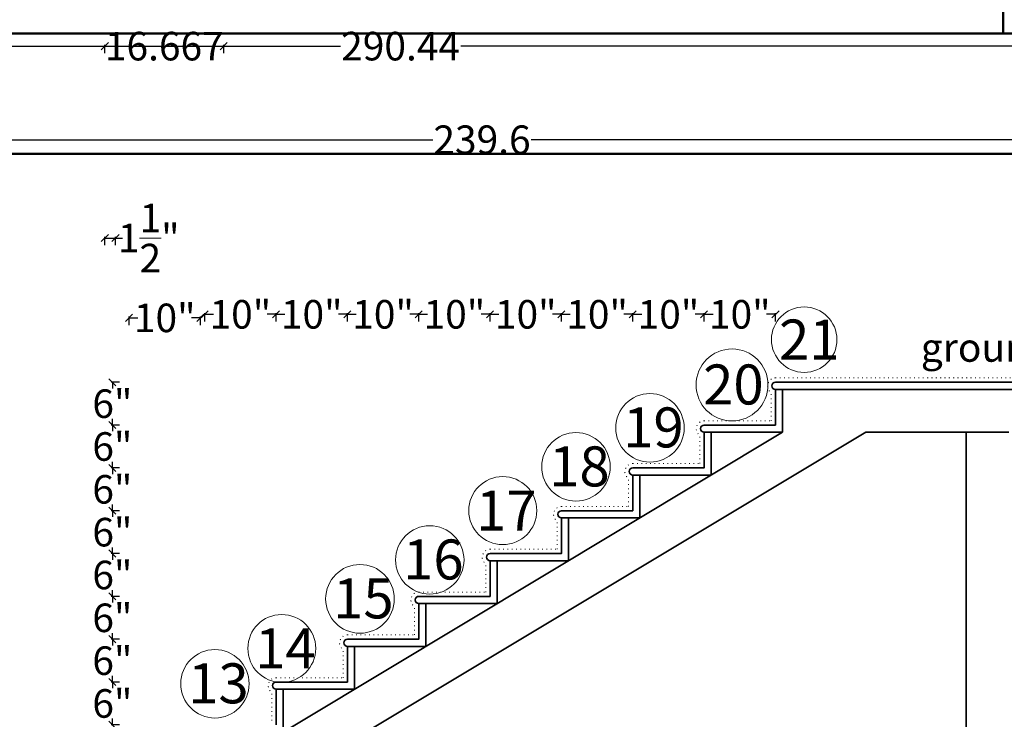
# Model space of a CAD drawing. Units: inches. Extents: x -60 to 284, y -245 to 257.
# Tile 4 of 10: x 55 to 193, y -86 to 12. Entities that reach past the tile are written whole.
import ezdxf

# ---------------------------------------------------------------- set-up
doc = ezdxf.new("R2010")
doc.units = ezdxf.units.IN
doc.header["$LTSCALE"] = 0.8
doc.header["$MEASUREMENT"] = 0
doc.linetypes.add('DOT', pattern=[6.35, 0, -6.35])
for name, color, linetype, lineweight in [('A-ANNO-DIMS', 2, 'Continuous', 18), ('A-ANNO-SYMB', 3, 'Continuous', 18), ('A-ANNO-TEXT', 3, 'Continuous', 18), ('A-ANNO-TTLB', 7, 'Continuous', 50), ('A-SECT', 7, 'Continuous', 35), ('A-SECT-OVHD', 8, 'DOT', 18), ('A-WALL', 7, 'Continuous', 50)]:
    doc.layers.add(name, color=color, linetype=linetype, lineweight=lineweight)
doc.styles.get("Standard").update_dxf_attribs({"font": 'arial.ttf'})
doc.dimstyles.get("Standard").update_dxf_attribs({"dimtxt": 4, "dimasz": 1, "dimexe": 0.18, "dimexo": 0.0625, "dimgap": 0.09, "dimtad": 0, "dimtih": 1, "dimtoh": 1, "dimzin": 0, "dimdsep": 46, "dimlunit": 4, "dimtxsty": 'Standard', "dimblk": 'OBLIQUE', "dimcen": 0.09, "dimadec": 0, "dimazin": 0, "dimtfac": 1, "dimtofl": 0, "dimtmove": 0, "dimatfit": 3, "dimfxl": 1, "dimfxlon": 1, "dimtolj": 1, "dimtzin": 0, "dimarcsym": 0})

# ---------------------------------------------------------------- blocks, each defined once
blk = doc.blocks.new('_Oblique')
at = {"color": 0, "linetype": 'ByBlock', "lineweight": -2}
blk.add_line((-0.5, -0.5), (0.5, 0.5), dxfattribs=at)
blk = doc.blocks.new('*D51')
at = {"layer": 'A-ANNO-DIMS', "color": 0, "lineweight": -2, "ltscale": 0.8, "transparency": 16777216}
for p, q in [((81.01, -30.69), (81.01, -29.51)), ((81.01, -29.69), (82.26, -29.69)), ((91.01, -29.69), (89.77, -29.69)), ((91.01, -30.69), (91.01, -29.51))]:
    blk.add_line(p, q, dxfattribs=at)
at = {"layer": 'Defpoints', "color": 0, "ltscale": 0.8, "transparency": 16777216}
for p in [(91.01, -29.69), (81.01, -87.21), (91.01, -87.21)]:
    blk.add_point(p, dxfattribs=at)
at = {"layer": 'A-ANNO-DIMS', "color": 0, "lineweight": -2, "ltscale": 0.8, "transparency": 16777216, "rotation": 180}
blk.add_blockref('_Oblique', (81.01, -29.69), dxfattribs=at)
at = {"layer": 'A-ANNO-DIMS', "color": 0, "lineweight": -2, "ltscale": 0.8, "transparency": 16777216}
blk.add_blockref('_Oblique', (91.01, -29.69), dxfattribs=at)
at = {"layer": 'A-ANNO-DIMS', "color": 0, "ltscale": 0.8, "transparency": 16777216, "insert": (86.01, -29.69), "char_height": 4, "attachment_point": 5}
blk.add_mtext('\\A1;10"', dxfattribs=at)
blk = doc.blocks.new('*D52')
at = {"layer": 'A-ANNO-DIMS', "color": 0, "lineweight": -2, "ltscale": 0.8, "transparency": 16777216}
for p, q in [((91.01, -30.69), (91.01, -29.51)), ((91.01, -29.69), (92.26, -29.69)), ((101.01, -29.69), (99.77, -29.69)), ((101.01, -30.69), (101.01, -29.51))]:
    blk.add_line(p, q, dxfattribs=at)
at = {"layer": 'Defpoints', "color": 0, "ltscale": 0.8, "transparency": 16777216}
for p in [(101.01, -29.69), (91.01, -81.21), (101.01, -81.21)]:
    blk.add_point(p, dxfattribs=at)
at = {"layer": 'A-ANNO-DIMS', "color": 0, "lineweight": -2, "ltscale": 0.8, "transparency": 16777216, "rotation": 180}
blk.add_blockref('_Oblique', (91.01, -29.69), dxfattribs=at)
at = {"layer": 'A-ANNO-DIMS', "color": 0, "lineweight": -2, "ltscale": 0.8, "transparency": 16777216}
blk.add_blockref('_Oblique', (101.01, -29.69), dxfattribs=at)
at = {"layer": 'A-ANNO-DIMS', "color": 0, "ltscale": 0.8, "transparency": 16777216, "insert": (96.01, -29.69), "char_height": 4, "attachment_point": 5}
blk.add_mtext('\\A1;10"', dxfattribs=at)
blk = doc.blocks.new('*D53')
at = {"layer": 'A-ANNO-DIMS', "color": 0, "lineweight": -2, "ltscale": 0.8, "transparency": 16777216}
for p, q in [((101.01, -30.69), (101.01, -29.51)), ((101.01, -29.69), (102.26, -29.69)), ((111.01, -29.69), (109.77, -29.69)), ((111.01, -30.69), (111.01, -29.51))]:
    blk.add_line(p, q, dxfattribs=at)
at = {"layer": 'Defpoints', "color": 0, "ltscale": 0.8, "transparency": 16777216}
for p in [(111.01, -29.69), (101.01, -75.21), (111.01, -75.21)]:
    blk.add_point(p, dxfattribs=at)
at = {"layer": 'A-ANNO-DIMS', "color": 0, "lineweight": -2, "ltscale": 0.8, "transparency": 16777216, "rotation": 180}
blk.add_blockref('_Oblique', (101.01, -29.69), dxfattribs=at)
at = {"layer": 'A-ANNO-DIMS', "color": 0, "lineweight": -2, "ltscale": 0.8, "transparency": 16777216}
blk.add_blockref('_Oblique', (111.01, -29.69), dxfattribs=at)
at = {"layer": 'A-ANNO-DIMS', "color": 0, "ltscale": 0.8, "transparency": 16777216, "insert": (106.01, -29.69), "char_height": 4, "attachment_point": 5}
blk.add_mtext('\\A1;10"', dxfattribs=at)
blk = doc.blocks.new('*D54')
at = {"layer": 'A-ANNO-DIMS', "color": 0, "lineweight": -2, "ltscale": 0.8, "transparency": 16777216}
for p, q in [((111.01, -30.69), (111.01, -29.51)), ((111.01, -29.69), (112.26, -29.69)), ((121.01, -29.69), (119.77, -29.69)), ((121.01, -30.69), (121.01, -29.51))]:
    blk.add_line(p, q, dxfattribs=at)
at = {"layer": 'Defpoints', "color": 0, "ltscale": 0.8, "transparency": 16777216}
for p in [(121.01, -29.69), (111.01, -69.21), (121.01, -69.21)]:
    blk.add_point(p, dxfattribs=at)
at = {"layer": 'A-ANNO-DIMS', "color": 0, "lineweight": -2, "ltscale": 0.8, "transparency": 16777216, "rotation": 180}
blk.add_blockref('_Oblique', (111.01, -29.69), dxfattribs=at)
at = {"layer": 'A-ANNO-DIMS', "color": 0, "lineweight": -2, "ltscale": 0.8, "transparency": 16777216}
blk.add_blockref('_Oblique', (121.01, -29.69), dxfattribs=at)
at = {"layer": 'A-ANNO-DIMS', "color": 0, "ltscale": 0.8, "transparency": 16777216, "insert": (116.01, -29.69), "char_height": 4, "attachment_point": 5}
blk.add_mtext('\\A1;10"', dxfattribs=at)
blk = doc.blocks.new('*D55')
at = {"layer": 'A-ANNO-DIMS', "color": 0, "lineweight": -2, "ltscale": 0.8, "transparency": 16777216}
for p, q in [((121.01, -30.69), (121.01, -29.51)), ((121.01, -29.69), (122.26, -29.69)), ((131.01, -29.69), (129.77, -29.69)), ((131.01, -30.69), (131.01, -29.51))]:
    blk.add_line(p, q, dxfattribs=at)
at = {"layer": 'Defpoints', "color": 0, "ltscale": 0.8, "transparency": 16777216}
for p in [(131.01, -29.69), (121.01, -63.21), (131.01, -63.21)]:
    blk.add_point(p, dxfattribs=at)
at = {"layer": 'A-ANNO-DIMS', "color": 0, "lineweight": -2, "ltscale": 0.8, "transparency": 16777216, "rotation": 180}
blk.add_blockref('_Oblique', (121.01, -29.69), dxfattribs=at)
at = {"layer": 'A-ANNO-DIMS', "color": 0, "lineweight": -2, "ltscale": 0.8, "transparency": 16777216}
blk.add_blockref('_Oblique', (131.01, -29.69), dxfattribs=at)
at = {"layer": 'A-ANNO-DIMS', "color": 0, "ltscale": 0.8, "transparency": 16777216, "insert": (126.01, -29.69), "char_height": 4, "attachment_point": 5}
blk.add_mtext('\\A1;10"', dxfattribs=at)
blk = doc.blocks.new('*D56')
at = {"layer": 'A-ANNO-DIMS', "color": 0, "lineweight": -2, "ltscale": 0.8, "transparency": 16777216}
for p, q in [((131.01, -30.69), (131.01, -29.51)), ((131.01, -29.69), (132.26, -29.69)), ((141.01, -29.69), (139.77, -29.69)), ((141.01, -30.69), (141.01, -29.51))]:
    blk.add_line(p, q, dxfattribs=at)
at = {"layer": 'Defpoints', "color": 0, "ltscale": 0.8, "transparency": 16777216}
for p in [(141.01, -29.69), (131.01, -57.21), (141.01, -57.21)]:
    blk.add_point(p, dxfattribs=at)
at = {"layer": 'A-ANNO-DIMS', "color": 0, "lineweight": -2, "ltscale": 0.8, "transparency": 16777216, "rotation": 180}
blk.add_blockref('_Oblique', (131.01, -29.69), dxfattribs=at)
at = {"layer": 'A-ANNO-DIMS', "color": 0, "lineweight": -2, "ltscale": 0.8, "transparency": 16777216}
blk.add_blockref('_Oblique', (141.01, -29.69), dxfattribs=at)
at = {"layer": 'A-ANNO-DIMS', "color": 0, "ltscale": 0.8, "transparency": 16777216, "insert": (136.01, -29.69), "char_height": 4, "attachment_point": 5}
blk.add_mtext('\\A1;10"', dxfattribs=at)
blk = doc.blocks.new('*D57')
at = {"layer": 'A-ANNO-DIMS', "color": 0, "lineweight": -2, "ltscale": 0.8, "transparency": 16777216}
for p, q in [((141.01, -30.69), (141.01, -29.51)), ((141.01, -29.69), (142.26, -29.69)), ((151.01, -29.69), (149.77, -29.69)), ((151.01, -30.69), (151.01, -29.51))]:
    blk.add_line(p, q, dxfattribs=at)
at = {"layer": 'Defpoints', "color": 0, "ltscale": 0.8, "transparency": 16777216}
for p in [(151.01, -29.69), (141.01, -51.21), (151.01, -51.21)]:
    blk.add_point(p, dxfattribs=at)
at = {"layer": 'A-ANNO-DIMS', "color": 0, "lineweight": -2, "ltscale": 0.8, "transparency": 16777216, "rotation": 180}
blk.add_blockref('_Oblique', (141.01, -29.69), dxfattribs=at)
at = {"layer": 'A-ANNO-DIMS', "color": 0, "lineweight": -2, "ltscale": 0.8, "transparency": 16777216}
blk.add_blockref('_Oblique', (151.01, -29.69), dxfattribs=at)
at = {"layer": 'A-ANNO-DIMS', "color": 0, "ltscale": 0.8, "transparency": 16777216, "insert": (146.01, -29.69), "char_height": 4, "attachment_point": 5}
blk.add_mtext('\\A1;10"', dxfattribs=at)
blk = doc.blocks.new('*D58')
at = {"layer": 'A-ANNO-DIMS', "color": 0, "lineweight": -2, "ltscale": 0.8, "transparency": 16777216}
for p, q in [((151.01, -30.69), (151.01, -29.51)), ((151.01, -29.69), (152.26, -29.69)), ((161.01, -29.69), (159.77, -29.69)), ((161.01, -30.69), (161.01, -29.51))]:
    blk.add_line(p, q, dxfattribs=at)
at = {"layer": 'Defpoints', "color": 0, "ltscale": 0.8, "transparency": 16777216}
for p in [(161.01, -29.69), (151.01, -45.21), (161.01, -45.21)]:
    blk.add_point(p, dxfattribs=at)
at = {"layer": 'A-ANNO-DIMS', "color": 0, "lineweight": -2, "ltscale": 0.8, "transparency": 16777216, "rotation": 180}
blk.add_blockref('_Oblique', (151.01, -29.69), dxfattribs=at)
at = {"layer": 'A-ANNO-DIMS', "color": 0, "lineweight": -2, "ltscale": 0.8, "transparency": 16777216}
blk.add_blockref('_Oblique', (161.01, -29.69), dxfattribs=at)
at = {"layer": 'A-ANNO-DIMS', "color": 0, "ltscale": 0.8, "transparency": 16777216, "insert": (156.01, -29.69), "char_height": 4, "attachment_point": 5}
blk.add_mtext('\\A1;10"', dxfattribs=at)
blk = doc.blocks.new('*D60')
at = {"layer": 'A-ANNO-DIMS', "color": 0, "lineweight": -2, "ltscale": 0.8, "transparency": 16777216}
for p, q in [((69.07, -81.21), (67.89, -81.21)), ((68.07, -81.21), (68.07, -82.08)), ((68.07, -87.21), (68.07, -86.34)), ((69.07, -87.21), (67.89, -87.21))]:
    blk.add_line(p, q, dxfattribs=at)
at = {"layer": 'Defpoints', "color": 0, "ltscale": 0.8, "transparency": 16777216}
for p in [(68.07, -81.21), (91.01, -81.21), (91.01, -87.21)]:
    blk.add_point(p, dxfattribs=at)
at = {"layer": 'A-ANNO-DIMS', "color": 0, "lineweight": -2, "ltscale": 0.8, "transparency": 16777216}
for p, rotation in [((68.07, -81.21), 90), ((68.07, -87.21), 270)]:
    blk.add_blockref('_Oblique', p, dxfattribs=dict(at, rotation=rotation))
at = {"layer": 'A-ANNO-DIMS', "color": 0, "ltscale": 0.8, "transparency": 16777216, "insert": (68.07, -84.21), "char_height": 4, "attachment_point": 5}
blk.add_mtext('\\A1;6"', dxfattribs=at)
blk = doc.blocks.new('*D61')
at = {"layer": 'A-ANNO-DIMS', "color": 0, "lineweight": -2, "ltscale": 0.8, "transparency": 16777216}
for p, q in [((69.07, -75.21), (67.89, -75.21)), ((68.07, -75.21), (68.07, -76.08)), ((69.07, -81.21), (67.89, -81.21)), ((68.07, -81.21), (68.07, -80.34))]:
    blk.add_line(p, q, dxfattribs=at)
at = {"layer": 'Defpoints', "color": 0, "ltscale": 0.8, "transparency": 16777216}
for p in [(68.07, -75.21), (101.01, -75.21), (101.01, -81.21)]:
    blk.add_point(p, dxfattribs=at)
at = {"layer": 'A-ANNO-DIMS', "color": 0, "lineweight": -2, "ltscale": 0.8, "transparency": 16777216}
for p, rotation in [((68.07, -75.21), 90), ((68.07, -81.21), 270)]:
    blk.add_blockref('_Oblique', p, dxfattribs=dict(at, rotation=rotation))
at = {"layer": 'A-ANNO-DIMS', "color": 0, "ltscale": 0.8, "transparency": 16777216, "insert": (68.07, -78.21), "char_height": 4, "attachment_point": 5}
blk.add_mtext('\\A1;6"', dxfattribs=at)
blk = doc.blocks.new('*D62')
at = {"layer": 'A-ANNO-DIMS', "color": 0, "lineweight": -2, "ltscale": 0.8, "transparency": 16777216}
for p, q in [((69.07, -69.21), (67.89, -69.21)), ((68.07, -69.21), (68.07, -70.08)), ((68.07, -75.21), (68.07, -74.34)), ((69.07, -75.21), (67.89, -75.21))]:
    blk.add_line(p, q, dxfattribs=at)
at = {"layer": 'Defpoints', "color": 0, "ltscale": 0.8, "transparency": 16777216}
for p in [(68.07, -69.21), (111.01, -69.21), (111.01, -75.21)]:
    blk.add_point(p, dxfattribs=at)
at = {"layer": 'A-ANNO-DIMS', "color": 0, "lineweight": -2, "ltscale": 0.8, "transparency": 16777216}
for p, rotation in [((68.07, -69.21), 90), ((68.07, -75.21), 270)]:
    blk.add_blockref('_Oblique', p, dxfattribs=dict(at, rotation=rotation))
at = {"layer": 'A-ANNO-DIMS', "color": 0, "ltscale": 0.8, "transparency": 16777216, "insert": (68.07, -72.21), "char_height": 4, "attachment_point": 5}
blk.add_mtext('\\A1;6"', dxfattribs=at)
blk = doc.blocks.new('*D63')
at = {"layer": 'A-ANNO-DIMS', "color": 0, "lineweight": -2, "ltscale": 0.8, "transparency": 16777216}
for p, q in [((69.07, -63.21), (67.89, -63.21)), ((68.07, -63.21), (68.07, -64.08)), ((68.07, -69.21), (68.07, -68.34)), ((69.07, -69.21), (67.89, -69.21))]:
    blk.add_line(p, q, dxfattribs=at)
at = {"layer": 'Defpoints', "color": 0, "ltscale": 0.8, "transparency": 16777216}
for p in [(68.07, -63.21), (121.01, -63.21), (121.01, -69.21)]:
    blk.add_point(p, dxfattribs=at)
at = {"layer": 'A-ANNO-DIMS', "color": 0, "lineweight": -2, "ltscale": 0.8, "transparency": 16777216}
for p, rotation in [((68.07, -63.21), 90), ((68.07, -69.21), 270)]:
    blk.add_blockref('_Oblique', p, dxfattribs=dict(at, rotation=rotation))
at = {"layer": 'A-ANNO-DIMS', "color": 0, "ltscale": 0.8, "transparency": 16777216, "insert": (68.07, -66.21), "char_height": 4, "attachment_point": 5}
blk.add_mtext('\\A1;6"', dxfattribs=at)
blk = doc.blocks.new('*D64')
at = {"layer": 'A-ANNO-DIMS', "color": 0, "lineweight": -2, "ltscale": 0.8, "transparency": 16777216}
for p, q in [((69.07, -57.21), (67.89, -57.21)), ((68.07, -57.21), (68.07, -58.08)), ((69.07, -63.21), (67.89, -63.21)), ((68.07, -63.21), (68.07, -62.34))]:
    blk.add_line(p, q, dxfattribs=at)
at = {"layer": 'Defpoints', "color": 0, "ltscale": 0.8, "transparency": 16777216}
for p in [(68.07, -57.21), (131.01, -57.21), (131.01, -63.21)]:
    blk.add_point(p, dxfattribs=at)
at = {"layer": 'A-ANNO-DIMS', "color": 0, "lineweight": -2, "ltscale": 0.8, "transparency": 16777216}
for p, rotation in [((68.07, -57.21), 90), ((68.07, -63.21), 270)]:
    blk.add_blockref('_Oblique', p, dxfattribs=dict(at, rotation=rotation))
at = {"layer": 'A-ANNO-DIMS', "color": 0, "ltscale": 0.8, "transparency": 16777216, "insert": (68.07, -60.21), "char_height": 4, "attachment_point": 5}
blk.add_mtext('\\A1;6"', dxfattribs=at)
blk = doc.blocks.new('*D65')
at = {"layer": 'A-ANNO-DIMS', "color": 0, "lineweight": -2, "ltscale": 0.8, "transparency": 16777216}
for p, q in [((69.07, -51.21), (67.89, -51.21)), ((68.07, -51.21), (68.07, -52.08)), ((68.07, -57.21), (68.07, -56.34)), ((69.07, -57.21), (67.89, -57.21))]:
    blk.add_line(p, q, dxfattribs=at)
at = {"layer": 'Defpoints', "color": 0, "ltscale": 0.8, "transparency": 16777216}
for p in [(68.07, -51.21), (141.01, -51.21), (141.01, -57.21)]:
    blk.add_point(p, dxfattribs=at)
at = {"layer": 'A-ANNO-DIMS', "color": 0, "lineweight": -2, "ltscale": 0.8, "transparency": 16777216}
for p, rotation in [((68.07, -51.21), 90), ((68.07, -57.21), 270)]:
    blk.add_blockref('_Oblique', p, dxfattribs=dict(at, rotation=rotation))
at = {"layer": 'A-ANNO-DIMS', "color": 0, "ltscale": 0.8, "transparency": 16777216, "insert": (68.07, -54.21), "char_height": 4, "attachment_point": 5}
blk.add_mtext('\\A1;6"', dxfattribs=at)
blk = doc.blocks.new('*D66')
at = {"layer": 'A-ANNO-DIMS', "color": 0, "lineweight": -2, "ltscale": 0.8, "transparency": 16777216}
for p, q in [((69.07, -45.21), (67.89, -45.21)), ((68.07, -45.21), (68.07, -46.08)), ((68.07, -51.21), (68.07, -50.34)), ((69.07, -51.21), (67.89, -51.21))]:
    blk.add_line(p, q, dxfattribs=at)
at = {"layer": 'Defpoints', "color": 0, "ltscale": 0.8, "transparency": 16777216}
for p in [(68.07, -45.21), (151.01, -45.21), (151.01, -51.21)]:
    blk.add_point(p, dxfattribs=at)
at = {"layer": 'A-ANNO-DIMS', "color": 0, "lineweight": -2, "ltscale": 0.8, "transparency": 16777216}
for p, rotation in [((68.07, -45.21), 90), ((68.07, -51.21), 270)]:
    blk.add_blockref('_Oblique', p, dxfattribs=dict(at, rotation=rotation))
at = {"layer": 'A-ANNO-DIMS', "color": 0, "ltscale": 0.8, "transparency": 16777216, "insert": (68.07, -48.21), "char_height": 4, "attachment_point": 5}
blk.add_mtext('\\A1;6"', dxfattribs=at)
blk = doc.blocks.new('*D67')
at = {"layer": 'A-ANNO-DIMS', "color": 0, "lineweight": -2, "ltscale": 0.8, "transparency": 16777216}
for p, q in [((69.07, -39.21), (67.89, -39.21)), ((68.07, -39.21), (68.07, -40.08)), ((69.07, -45.21), (67.89, -45.21)), ((68.07, -45.21), (68.07, -44.34))]:
    blk.add_line(p, q, dxfattribs=at)
at = {"layer": 'Defpoints', "color": 0, "ltscale": 0.8, "transparency": 16777216}
for p in [(68.07, -39.21), (161.01, -39.21), (161.01, -45.21)]:
    blk.add_point(p, dxfattribs=at)
at = {"layer": 'A-ANNO-DIMS', "color": 0, "lineweight": -2, "ltscale": 0.8, "transparency": 16777216}
for p, rotation in [((68.07, -39.21), 90), ((68.07, -45.21), 270)]:
    blk.add_blockref('_Oblique', p, dxfattribs=dict(at, rotation=rotation))
at = {"layer": 'A-ANNO-DIMS', "color": 0, "ltscale": 0.8, "transparency": 16777216, "insert": (68.07, -42.21), "char_height": 4, "attachment_point": 5}
blk.add_mtext('\\A1;6"', dxfattribs=at)
blk = doc.blocks.new('*D72')
at = {"layer": 'A-ANNO-DIMS', "color": 0, "lineweight": -2, "ltscale": 0.8, "transparency": 16777216}
for p, q in [((67.01, -20.01), (67.01, -18.83)), ((67.01, -19.01), (68.51, -19.01)), ((68.51, -20.01), (68.51, -18.83)), ((68.51, -19.01), (69.51, -19.01))]:
    blk.add_line(p, q, dxfattribs=at)
at = {"layer": 'Defpoints', "color": 0, "ltscale": 0.8, "transparency": 16777216}
for p in [(68.51, -19.01), (67.01, -93.21), (68.51, -93.21)]:
    blk.add_point(p, dxfattribs=at)
at = {"layer": 'A-ANNO-DIMS', "color": 0, "lineweight": -2, "ltscale": 0.8, "transparency": 16777216, "rotation": 180}
blk.add_blockref('_Oblique', (67.01, -19.01), dxfattribs=at)
at = {"layer": 'A-ANNO-DIMS', "color": 0, "lineweight": -2, "ltscale": 0.8, "transparency": 16777216}
blk.add_blockref('_Oblique', (68.51, -19.01), dxfattribs=at)
at = {"layer": 'A-ANNO-DIMS', "color": 0, "ltscale": 0.8, "transparency": 16777216, "insert": (73.17, -19.01), "char_height": 4, "attachment_point": 5}
blk.add_mtext('\\A1;1{\\H1x;\\S1/2;}"', dxfattribs=at)
blk = doc.blocks.new('*D73')
at = {"layer": 'A-ANNO-DIMS', "color": 0, "lineweight": -2, "ltscale": 0.8, "transparency": 16777216}
for p, q in [((70.41, -31.19), (70.41, -30.01)), ((70.41, -30.19), (71.66, -30.19)), ((80.41, -30.19), (79.17, -30.19)), ((80.41, -31.19), (80.41, -30.01))]:
    blk.add_line(p, q, dxfattribs=at)
at = {"layer": 'Defpoints', "color": 0, "ltscale": 0.8, "transparency": 16777216}
for p in [(80.41, -30.19), (70.41, -93.21), (80.41, -93.21)]:
    blk.add_point(p, dxfattribs=at)
at = {"layer": 'A-ANNO-DIMS', "color": 0, "lineweight": -2, "ltscale": 0.8, "transparency": 16777216, "rotation": 180}
blk.add_blockref('_Oblique', (70.41, -30.19), dxfattribs=at)
at = {"layer": 'A-ANNO-DIMS', "color": 0, "lineweight": -2, "ltscale": 0.8, "transparency": 16777216}
blk.add_blockref('_Oblique', (80.41, -30.19), dxfattribs=at)
at = {"layer": 'A-ANNO-DIMS', "color": 0, "ltscale": 0.8, "transparency": 16777216, "insert": (75.41, -30.19), "char_height": 4, "attachment_point": 5}
blk.add_mtext('\\A1;10"', dxfattribs=at)
blk = doc.blocks.new('*D89')
at = {"layer": 'A-ANNO-DIMS', "color": 0, "lineweight": -2, "ltscale": 0.8, "transparency": 16777216}
for p, q in [((0.09, -4.23), (0.09, -5.41)), ((0.09, -5.23), (113, -5.23)), ((239.66, -5.23), (126.75, -5.23)), ((239.66, -4.23), (239.66, -5.41))]:
    blk.add_line(p, q, dxfattribs=at)
at = {"layer": 'Defpoints', "color": 0, "ltscale": 0.8, "transparency": 16777216}
for p in [(0.09, 9.67), (239.66, 9.67), (239.66, -5.23)]:
    blk.add_point(p, dxfattribs=at)
at = {"layer": 'A-ANNO-DIMS', "color": 0, "lineweight": -2, "ltscale": 0.8, "transparency": 16777216, "rotation": 180}
blk.add_blockref('_Oblique', (0.09, -5.23), dxfattribs=at)
at = {"layer": 'A-ANNO-DIMS', "color": 0, "lineweight": -2, "ltscale": 0.8, "transparency": 16777216}
blk.add_blockref('_Oblique', (239.66, -5.23), dxfattribs=at)
at = {"layer": 'A-ANNO-DIMS', "color": 0, "ltscale": 0.8, "transparency": 16777216, "insert": (119.88, -5.23), "char_height": 4, "attachment_point": 5}
blk.add_mtext('\\A1;239.6', dxfattribs=at)
blk = doc.blocks.new('*D111')
at = {"layer": 'A-ANNO-DIMS', "color": 0, "lineweight": -2, "ltscale": 0.8, "transparency": 16777216}
for p, q in [((-50.85, -46.21), (-52.03, -46.21)), ((-51.85, -46.21), (-51.85, -49.97)), ((-51.85, -57.93), (-51.85, -54.17)), ((-50.85, -57.93), (-52.03, -57.93))]:
    blk.add_line(p, q, dxfattribs=at)
at = {"layer": 'Defpoints', "color": 0, "ltscale": 0.8, "transparency": 16777216}
for p in [(193.74, -46.21), (-51.85, -57.93), (193.74, -57.93)]:
    blk.add_point(p, dxfattribs=at)
at = {"layer": 'A-ANNO-DIMS', "color": 0, "lineweight": -2, "ltscale": 0.8, "transparency": 16777216}
for p, rotation in [((-51.85, -46.21), 90), ((-51.85, -57.93), 270)]:
    blk.add_blockref('_Oblique', p, dxfattribs=dict(at, rotation=rotation))
at = {"layer": 'A-ANNO-DIMS', "color": 0, "ltscale": 0.8, "transparency": 16777216, "insert": (-51.85, -52.07), "char_height": 4, "attachment_point": 5}
blk.add_mtext('\\A1;11.717', dxfattribs=at)
blk = doc.blocks.new('*D113')
at = {"layer": 'A-ANNO-DIMS', "color": 0, "lineweight": -2, "ltscale": 0.8, "transparency": 16777216}
for p, q in [((67.01, 6.88), (67.01, 8.06)), ((67.01, 7.88), (67.14, 7.88)), ((83.68, 7.88), (83.55, 7.88)), ((83.68, 6.88), (83.68, 8.06))]:
    blk.add_line(p, q, dxfattribs=at)
at = {"layer": 'Defpoints', "color": 0, "ltscale": 0.8, "transparency": 16777216}
for p in [(83.68, 7.88), (67.01, -93.21), (83.68, -93.21)]:
    blk.add_point(p, dxfattribs=at)
at = {"layer": 'A-ANNO-DIMS', "color": 0, "lineweight": -2, "ltscale": 0.8, "transparency": 16777216, "rotation": 180}
blk.add_blockref('_Oblique', (67.01, 7.88), dxfattribs=at)
at = {"layer": 'A-ANNO-DIMS', "color": 0, "lineweight": -2, "ltscale": 0.8, "transparency": 16777216}
blk.add_blockref('_Oblique', (83.68, 7.88), dxfattribs=at)
at = {"layer": 'A-ANNO-DIMS', "color": 0, "ltscale": 0.8, "transparency": 16777216, "insert": (75.35, 7.88), "char_height": 4, "attachment_point": 5}
blk.add_mtext('\\A1;16.667', dxfattribs=at)
blk = doc.blocks.new('*D114')
at = {"layer": 'A-ANNO-DIMS', "color": 0, "lineweight": -2, "ltscale": 0.8, "transparency": 16777216}
for p, q in [((-36.75, 6.88), (-36.75, 8.06)), ((-36.75, 7.88), (100.05, 7.88)), ((253.69, 7.88), (116.89, 7.88)), ((253.69, 6.88), (253.69, 8.06))]:
    blk.add_line(p, q, dxfattribs=at)
at = {"layer": 'Defpoints', "color": 0, "ltscale": 0.8, "transparency": 16777216}
for p in [(253.69, 7.88), (-36.75, -7.22), (253.69, -7.22)]:
    blk.add_point(p, dxfattribs=at)
at = {"layer": 'A-ANNO-DIMS', "color": 0, "lineweight": -2, "ltscale": 0.8, "transparency": 16777216, "rotation": 180}
blk.add_blockref('_Oblique', (-36.75, 7.88), dxfattribs=at)
at = {"layer": 'A-ANNO-DIMS', "color": 0, "lineweight": -2, "ltscale": 0.8, "transparency": 16777216}
blk.add_blockref('_Oblique', (253.69, 7.88), dxfattribs=at)
at = {"layer": 'A-ANNO-DIMS', "color": 0, "ltscale": 0.8, "transparency": 16777216, "insert": (108.47, 7.88), "char_height": 4, "attachment_point": 5}
blk.add_mtext('\\A1;290.44', dxfattribs=at)

msp = doc.modelspace()

# ---------------------------------------------------------------- linework, layer by layer
at = {"layer": 'A-ANNO-SYMB', "ltscale": 0.8}
for centre, radius in [((165.0409, -33.2357), 4.5856), ((154.9236, -39.5809), 5.0387), ((143.4181, -45.5984), 4.8002), ((133.0495, -51.0562), 4.8002), ((122.7935, -57.193), 4.7667), ((112.5631, -64.098), 4.7941), ((102.778, -69.5557), 4.8123), ((91.8165, -76.5051), 4.7576), ((82.4403, -81.4528), 4.7968)]:
    msp.add_circle(centre, radius, dxfattribs=at)
at = {"layer": 'A-ANNO-TTLB', "ltscale": 0.8}
for points in [[(0.0867, 122.666), (239.6639, 122.666), (239.6639, 9.666), (0.0867, 9.666)], [(-36.7489, -7.223), (253.6882, -7.223), (253.6882, -227.2835), (-36.7489, -227.2835)]]:
    msp.add_lwpolyline(points, close=True, dxfattribs=at)
at = {"layer": 'A-SECT', "ltscale": 0.8}
for p, q in [((161.0139, -40.2089), (244.8977, -40.2089)), ((162.0139, -46.2089), (162.0139, -40.2089)), ((151.0139, -46.2089), (162.0139, -46.2089)), ((152.0139, -52.2089), (152.0139, -46.2089)), ((161.0139, -46.2089), (162.0139, -46.2089)), ((173.6758, -46.2089), (187.7426, -46.2089)), ((187.7426, -46.2089), (187.7426, -147.2089)), ((193.7426, -46.2089), (187.7426, -46.2089)), ((141.0139, -52.2089), (152.0139, -52.2089)), ((142.0139, -58.2089), (142.0139, -52.2089)), ((131.0139, -58.2089), (142.0139, -58.2089)), ((132.0139, -64.2089), (132.0139, -58.2089)), ((121.0139, -64.2089), (132.0139, -64.2089)), ((122.0139, -70.2089), (122.0139, -64.2089)), ((111.0139, -70.2089), (122.0139, -70.2089)), ((112.0139, -76.2089), (112.0139, -70.2089)), ((101.0139, -76.2089), (112.0139, -76.2089)), ((102.0139, -82.2089), (102.0139, -76.2089)), ((91.0139, -82.2089), (102.0139, -82.2089)), ((92.0139, -88.2089), (92.0139, -82.2089))]:
    msp.add_line(p, q, dxfattribs=at)
msp.add_lwpolyline([(91.0139, -87.2089), (91.0139, -82.2089, -1), (91.0139, -81.2089), (101.0139, -81.2089), (101.0139, -76.2089, -1), (101.0139, -75.2089), (111.0139, -75.2089), (111.0139, -70.2089, -1), (111.0139, -69.2089), (121.0139, -69.2089), (121.0139, -64.2089, -1), (121.0139, -63.2089), (131.0139, -63.2089), (131.0139, -58.2089, -1), (131.0139, -57.2089), (141.0139, -57.2089), (141.0139, -52.2089, -1), (141.0139, -51.2089), (151.0139, -51.2089), (151.0139, -46.2089, -1), (151.0139, -45.2089), (161.0139, -45.2089), (161.0139, -40.2089, -1), (161.0139, -39.2089), (244.8977, -39.2089)], format="xyb", dxfattribs=at)
for points in [[(162.0139, -46.2089), (83.6806, -93.2089)], [(173.6758, -46.2089), (86.557, -98.4801)]]:
    msp.add_lwpolyline(points, dxfattribs=at)
at = {"layer": 'A-SECT-OVHD', "ltscale": 0.1}
msp.add_lwpolyline([(90.4139, -86.6089), (90.4139, -82.6308, -0.74635672), (91.0139, -80.6089), (100.4139, -80.6089), (100.4139, -76.6308, -0.74635672), (101.0139, -74.6089), (110.4139, -74.6089), (110.4139, -70.6308, -0.74635672), (111.0139, -68.6089), (120.4139, -68.6089), (120.4139, -64.6308, -0.74635672), (121.0139, -62.6089), (130.4139, -62.6089), (130.4139, -58.6308, -0.74635672), (131.0139, -56.6089), (140.4139, -56.6089), (140.4139, -52.6308, -0.74635672), (141.0139, -50.6089), (150.4139, -50.6089), (150.4139, -46.6308, -0.74635672), (151.0139, -44.6089), (160.4139, -44.6089), (160.4139, -40.6308, -0.74635672), (161.0139, -38.6089), (244.8977, -38.6089)], format="xyb", dxfattribs=at)
at = {"layer": 'A-WALL'}
msp.add_lwpolyline([(192.9361, 9.666), (192.9361, 15.666), (159.9361, 15.666), (79.9361, 15.666), (37.9361, 15.666), (33.9361, 15.666), (33.9361, 9.666)], dxfattribs=at)

# ---------------------------------------------------------------- texts
at = {"layer": 'A-ANNO-TEXT', "ltscale": 0.8, "attachment_point": 1}
for s, width, gutter_width, insert, char_height in [('21', 28.020867, 2.8021, (161.5202, -30.4221), 5.60417), ('ground finish floor lvl +6\'-9"', 97.551324, 1, (181.3842, -32.3395), 4), ('20', 28.020867, 2.8021, (150.8714, -36.7196), 5.60417), ('19', 28.020867, 2.8021, (139.6622, -42.7371), 5.60417), ('18', 28.020867, 2.8021, (129.2937, -48.1949), 5.60417), ('17', 28.020867, 2.8021, (119.0433, -54.3794), 5.60417), ('16', 28.020867, 2.8021, (108.8149, -61.2366), 5.60417), ('15', 28.020867, 2.8021, (99.0068, -66.6944), 5.60417), ('14', 28.020867, 2.8021, (88.0778, -73.6916), 5.60417), ('13', 28.020867, 2.8021, (78.6901, -78.5896), 5.60417)]:
    msp.add_mtext_dynamic_manual_height_columns(s, width=width, gutter_width=gutter_width, heights=[0], dxfattribs=dict(at, insert=insert, char_height=char_height))

# ---------------------------------------------------------------- dimensions: what is measured, and where the dimension line sits
at = {"layer": 'A-ANNO-DIMS', "ltscale": 0.8}
for base, p1, p2, override, picture, middle in [((253.6882, 7.877), (-36.7489, -7.223), (253.6882, -7.223), {"dimdec": 2, "dimlfac": 1, "dimrnd": 0, "dimzin": 0, "dimdsep": 46, "dimlunit": 2}, '*D114', (108.4697, 7.877)), ((239.6639, -5.234), (0.0867, 9.666), (239.6639, 9.666), {"dimdec": 1, "dimlfac": 1, "dimrnd": 0, "dimzin": 0, "dimdsep": 46, "dimlunit": 2}, '*D89', (119.8753, -5.234)), ((83.6806, 7.877), (67.0139, -93.2089), (83.6806, -93.2089), {"dimdec": 3, "dimlfac": 1, "dimrnd": 0, "dimzin": 0, "dimdsep": 46, "dimlunit": 2}, '*D113', (75.3472, 7.877)), ((68.5139, -19.0057), (67.0139, -93.2089), (68.5139, -93.2089), {"dimclrd": 0, "dimclre": 0, "dimclrt": 0}, '*D72', (73.1728, -19.0057)), ((80.4139, -30.1873), (70.4139, -93.2089), (80.4139, -93.2089), {"dimclrd": 0, "dimclre": 0, "dimclrt": 0}, '*D73', (75.4139, -30.1873)), ((91.0139, -29.6873), (81.0139, -87.2089), (91.0139, -87.2089), {"dimclrd": 0, "dimclre": 0, "dimclrt": 0}, '*D51', (86.0139, -29.6873)), ((101.0139, -29.6873), (91.0139, -81.2089), (101.0139, -81.2089), {"dimclrd": 0, "dimclre": 0, "dimclrt": 0}, '*D52', (96.0139, -29.6873)), ((111.0139, -29.6873), (101.0139, -75.2089), (111.0139, -75.2089), {"dimclrd": 0, "dimclre": 0, "dimclrt": 0}, '*D53', (106.0139, -29.6873)), ((121.0139, -29.6873), (111.0139, -69.2089), (121.0139, -69.2089), {"dimclrd": 0, "dimclre": 0, "dimclrt": 0}, '*D54', (116.0139, -29.6873)), ((131.0139, -29.6873), (121.0139, -63.2089), (131.0139, -63.2089), {"dimclrd": 0, "dimclre": 0, "dimclrt": 0}, '*D55', (126.0139, -29.6873)), ((141.0139, -29.6873), (131.0139, -57.2089), (141.0139, -57.2089), {"dimclrd": 0, "dimclre": 0, "dimclrt": 0}, '*D56', (136.0139, -29.6873)), ((151.0139, -29.6873), (141.0139, -51.2089), (151.0139, -51.2089), {"dimclrd": 0, "dimclre": 0, "dimclrt": 0}, '*D57', (146.0139, -29.6873)), ((161.0139, -29.6873), (151.0139, -45.2089), (161.0139, -45.2089), {"dimclrd": 0, "dimclre": 0, "dimclrt": 0}, '*D58', (156.0139, -29.6873))]:
    dim = msp.add_linear_dim(base=base, p1=p1, p2=p2, dimstyle='Standard', override=override, dxfattribs=at)
    dim.commit()
    dim.dimension.update_dxf_attribs({"geometry": picture, "text_midpoint": middle})
for base, p1, p2, override, picture, middle in [((68.0702, -39.2089), (161.0139, -45.2089), (161.0139, -39.2089), {"dimclrd": 0, "dimclre": 0, "dimclrt": 0}, '*D67', (68.0702, -42.2089)), ((68.0702, -45.2089), (151.0139, -51.2089), (151.0139, -45.2089), {"dimclrd": 0, "dimclre": 0, "dimclrt": 0}, '*D66', (68.0702, -48.2089)), ((-51.8489, -57.9262), (193.7426, -46.2089), (193.7426, -57.9262), {"dimdec": 3, "dimlfac": 1, "dimrnd": 0, "dimzin": 0, "dimdsep": 46, "dimlunit": 2}, '*D111', (-51.8489, -52.0675)), ((68.0702, -51.2089), (141.0139, -57.2089), (141.0139, -51.2089), {"dimclrd": 0, "dimclre": 0, "dimclrt": 0}, '*D65', (68.0702, -54.2089)), ((68.0702, -57.2089), (131.0139, -63.2089), (131.0139, -57.2089), {"dimclrd": 0, "dimclre": 0, "dimclrt": 0}, '*D64', (68.0702, -60.2089)), ((68.0702, -63.2089), (121.0139, -69.2089), (121.0139, -63.2089), {"dimclrd": 0, "dimclre": 0, "dimclrt": 0}, '*D63', (68.0702, -66.2089)), ((68.0702, -69.2089), (111.0139, -75.2089), (111.0139, -69.2089), {"dimclrd": 0, "dimclre": 0, "dimclrt": 0}, '*D62', (68.0702, -72.2089)), ((68.0702, -75.2089), (101.0139, -81.2089), (101.0139, -75.2089), {"dimclrd": 0, "dimclre": 0, "dimclrt": 0}, '*D61', (68.0702, -78.2089)), ((68.0702, -81.2089), (91.0139, -87.2089), (91.0139, -81.2089), {"dimclrd": 0, "dimclre": 0, "dimclrt": 0}, '*D60', (68.0702, -84.2089))]:
    dim = msp.add_linear_dim(base=base, p1=p1, p2=p2, angle=90, dimstyle='Standard', override=override, dxfattribs=at)
    dim.commit()
    dim.dimension.update_dxf_attribs({"geometry": picture, "text_midpoint": middle})

doc.saveas('drawing.dxf')
